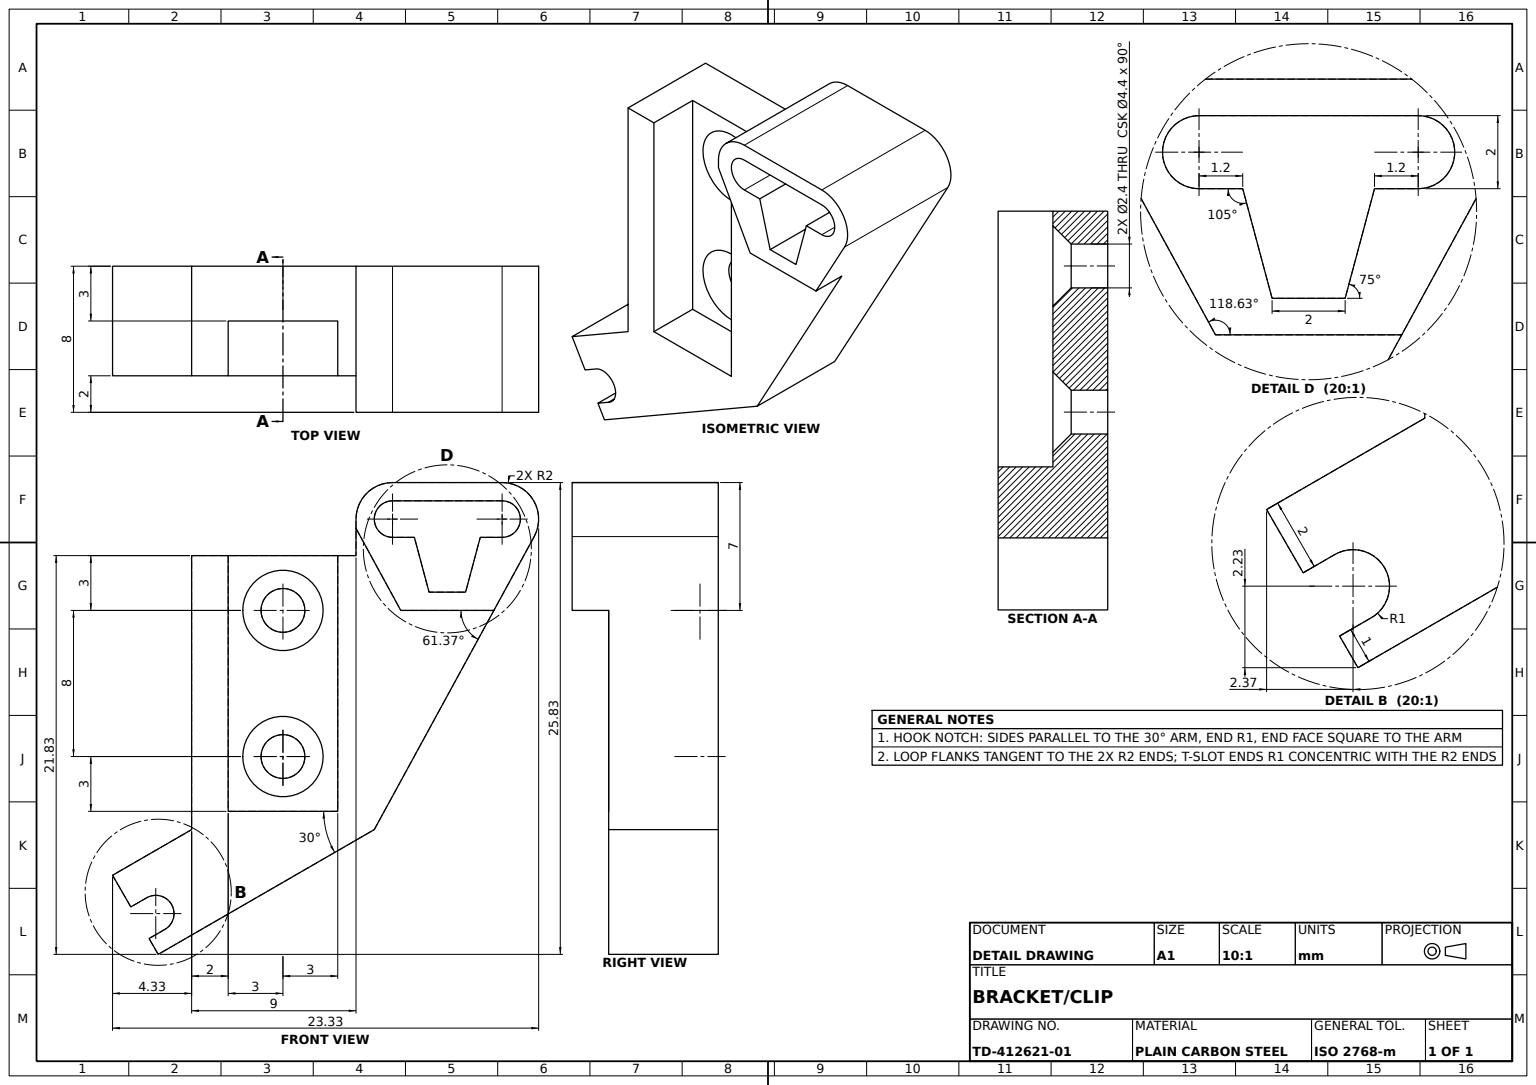
SolidWorks part; units mm, degrees
material "Plain Carbon Steel"
ref_plane "Front Plane" through (0, 0, 0) normal (0, 0, 1) x (1, 0, 0)
ref_plane "Top Plane" through (0, 0, 0) normal (0, 1, 0) x (1, 0, 0)
ref_plane "Right Plane" through (0, 0, 0) normal (1, 0, 0) x (0, 0, -1)
sketch "L Bracket Profile Sketch" plane through (0, 0, 0) normal (0, 0, 1) x (1, 0, 0)
  line L0 (0, 0) -> (0, 15)
  line L1 (0, 0) -> (-4.3301, -2.5)
  line L3 (10, 0) -> (-1.8301, -6.8301)
  line L4 (-4.3301, -2.5) -> (-3.3296, -4.233)
  line L5 (-1.8301, -6.8301) -> (-2.3307, -5.9631)
  line L6 (0, 15) -> (9, 15)
  line L7 (-1.5055, -5.4867) -> (-2.3307, -5.9631)
  line L8 (-2.5044, -3.7566) -> (-3.3296, -4.233)
  line L9 (-2.3307, -5.9631) -> (-1.8301, -6.8301)
  line L11 (9, 17) -> (9, 15)
  line L15 (11, 19) -> (17, 19)
  line L17 (18.7555, 16.0418) -> (10, 0)
  line L19 (13, 13) -> (15, 13)
  line L20 (15, 13) -> (15.8038, 16)
  line L21 (13, 13) -> (12.1962, 16)
  line L23 (9.2445, 16.0418) -> (11.4505, 12)
  line L24 (11, 18) -> (17, 18)
  line L25 (14, 12) -> (16.5495, 12)
  line L26 (14, 12) -> (11.4505, 12)
  line L27 (17, 16) -> (15.8038, 16)
  line L28 (12.1962, 16) -> (11, 16)
  arc A1 (-1.5055, -5.4867) -> (-2.5044, -3.7566) centre (-1.9641, -4.5981) ccw
  arc A6 (11, 19) -> (9.2445, 16.0418) centre (11, 17) ccw
  arc A7 (18.7555, 16.0418) -> (17, 19) centre (17, 17) ccw
  arc A8 (11, 18) -> (11, 16) centre (11, 17) ccw
  arc A9 (17, 16) -> (17, 18) centre (17, 17) ccw
  dimension "D1" = 2
  dimension "D2" = 2
  dimension "D4" = 1
  dimension "D15" = 1
  dimension "D3" = 1.9641
  dimension "D5" = 4.5981
  dimension "D6" = 2.0011
  dimension "D7" = 5
  dimension "D8" = 1
  dimension "D9" = 3.9989
  dimension "D10" = 18.2757
  dimension "D11" = 16.0418
  dimension "D12" = 8.7777
  dimension "D13" = 9
  dimension "D14" = 15
  dimension "D16" = 4.0418
  dimension "D17" = 5.0991
  dimension "D18" = 5
  dimension "D19" = 6
  dimension "D20" = 15
  dimension "D21" = 15.9217
  dimension "D22" = 11.1242
  dimension "D23" = 30
extrude "L Bracket Body" add sketch "L Bracket Profile Sketch" along normal blind 6 contours A6 L11 L6 L0 L1 L4 L8 A1 L7 L5 L3 L17 L25 L26 L23 | L17 A7 L15 A6 L23 L26 L25 A9 L27 L20 L19 L21 L28 A8 L24
sketch "Trapezoid Slot Boss Sketch" plane through (0, 0, 6) normal (0, 0, 1) x (1, 0, 0)
  line L0 (11, 18) -> (17, 18)
  line L2 (14, 12) -> (16.5495, 12)
  line L3 (11, 16) -> (12.1962, 16)
  line L4 (14, 12) -> (11.4505, 12)
  line L5 (16.5495, 12) -> (18.7555, 16.0418)
  line L6 (11.4505, 12) -> (9, 16.4897)
  line L7 (15.8038, 16) -> (15, 13)
  line L8 (15, 13) -> (13, 13)
  line L9 (13, 13) -> (12.1962, 16)
  line L10 (15.8038, 16) -> (17, 16)
  line L11 (10, 0) -> (18.7555, 16.0418)
  line L12 (17, 19) -> (11, 19)
  line L13 (9, 17) -> (9, 15)
  line L14 (9, 15) -> (0, 15)
  line L15 (0, 15) -> (0, 0)
  line L16 (0, 0) -> (-4.3301, -2.5)
  line L17 (-4.3301, -2.5) -> (-3.3296, -4.233)
  line L18 (-3.3296, -4.233) -> (-2.5044, -3.7566)
  line L19 (-1.5055, -5.4867) -> (-2.3307, -5.9631)
  line L20 (-2.3307, -5.9631) -> (-1.8301, -6.8301)
  line L21 (-1.8301, -6.8301) -> (10, 0)
  line L23 (17, 19) -> (11, 19)
  line L24 (9, 17) -> (9, 16.4897)
  arc A0 (17, 16) -> (17, 18) centre (17, 17) ccw
  arc A1 (11, 18) -> (11, 16) centre (11, 17) ccw
  arc A3 (18.7555, 16.0418) -> (17, 19) centre (17, 17) ccw
  arc A4 (11, 19) -> (9, 17) centre (11, 17) ccw
  arc A5 (-1.5055, -5.4867) -> (-2.5044, -3.7566) centre (-1.9641, -4.5981) ccw
  arc A6 (18.7555, 16.0418) -> (17, 19) centre (17, 17) ccw
  arc A7 (11, 19) -> (9, 17) centre (11, 17) ccw
  point P2 (14, 13)
  dimension "D2" = 4.0418
  dimension "D3" = 2.717
  dimension "D4" = 298.625
  dimension "D5" = 4.4897
  dimension "D6" = 14
  dimension "D1" = 0
extrude "Trapezoid Slot Boss" add sketch "Trapezoid Slot Boss Sketch" along normal blind 2
sketch "Pocket Cut Sketch" plane through (0, 15, 0) normal (0, 1, 0) x (1, 0, 0)
  line L0 (2, -6) -> (5, -6)
  line L1 (0, -6) -> (9, -6) construction
  line L3 (5, -3) -> (8, -3)
  line L4 (5, -3) -> (2, -3)
  line L5 (2, -3) -> (2, -6)
  line L6 (2, -6) -> (8, -6)
  line L7 (8, -6) -> (8, -3)
  line M7 (0, -6) -> (9, -6)
  dimension "D1" = 3
  dimension "D2" = 3
  dimension "D3" = 5
  dimension "D4" = 2
  dimension "D5" = 6
  dimension "D6" = 5
extrude "Pocket Cut" cut sketch "Pocket Cut Sketch" against normal blind 14 contours L7 L3 L4 L5 M7
hole_wizard "M2 Countersunk Holes" positions "Sketch4" profile "Sketch5" countersink size "M2" standard "ISO" end condition through all
sketch "Sketch4" plane through (0, 0, 3) normal (0, 0, 1) x (1, 0, 0)
  line L0 (2, 15) -> (8, 15) construction
  line L1 (2, 1) -> (2, 15) construction
  line L2 (2, 1) -> (8, 1) construction
  line L3 (2, 1) -> (2, 15) construction
  point P0 (5, 12)
  point P2 (5, 4)
  dimension "D1" = 3
  dimension "D2" = 3
  dimension "D3" = 3
  dimension "D4" = 3
sketch "Sketch5" plane through (5, 12, 3) normal (1, 0, 0) x (0, -1, 0)
  line L0 (0, 0) -> (0, 3)
  line L1 (0, 3) -> (1.2, 3)
  line L2 (1.2, 3) -> (1.2, 1)
  line L3 (1.2, 1) -> (2.2, 0)
  line L5 (2.2, 0) -> (0, 0)
  line L6 (-1.2, 1) -> (-2.2, 0) construction
  line L11 (0, -6.35) -> (0, 107.95) construction
  dimension "Thru Hole Dia." = 2.4
  dimension "Thru Hole Depth" = 3
  dimension "Near C'Sink Dia." = 4.4
  dimension "Near C'Sink Angle" = 90
